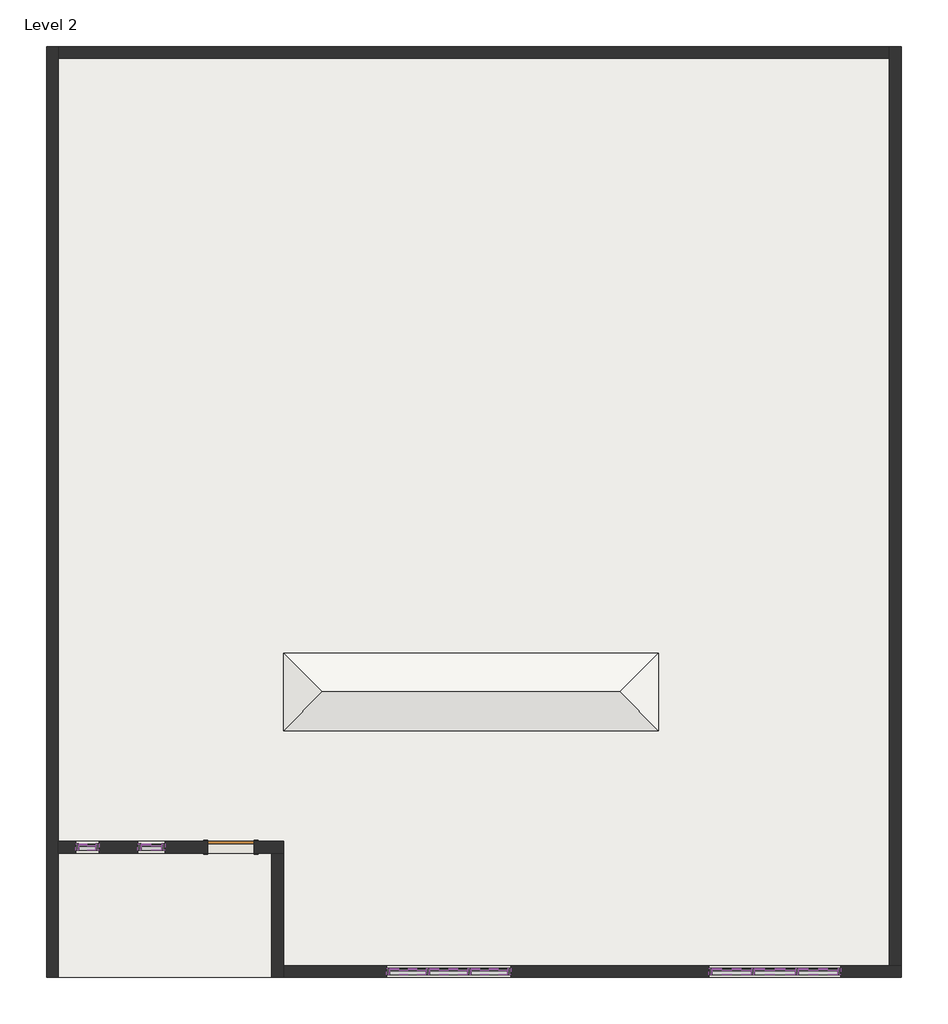
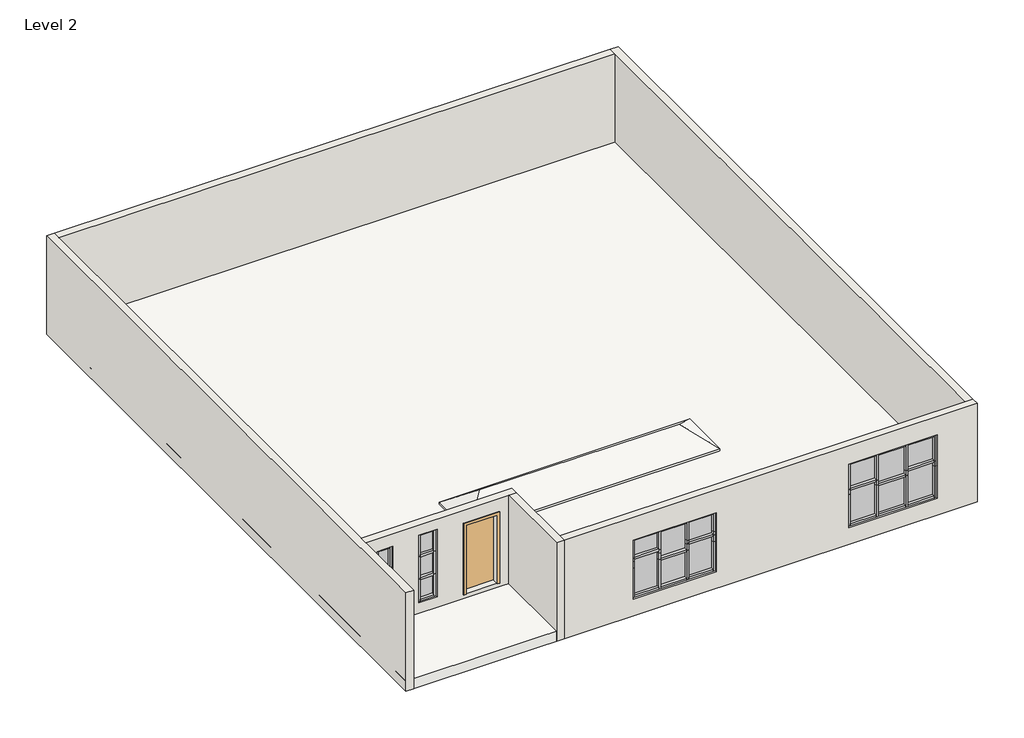
# One storey: 66 members, 18 plates, 6 walls, 2 roofs, 1 door.
"""IFC4 building model written with IfcOpenShell, lengths in millimetres."""

from ifc_helpers import new_model, si_unit, frame, origin, place, context, project, spatial, polyline, outline, extrude, faceted_brep, transform, mapped, element, save
from components import door_0ca8825f, member_ff9f2d30, member_0c1408be, member_7007ad49, member_abeaf8ac, member_9d02be77, member_798d6cad, member_f6f0dfdd, member_876f8f00, member_418a0375, member_7cfea1b5, member_90c805a2, member_80b47cb0, member_0b6e4484, member_4d11dfbc, member_589dede6, member_5e78fce7, member_cffb459a, member_c9167585, member_da94038d, member_275f0c90, member_171fbd6b, member_46f5bc36, member_7d5d45fc, member_9b02ea12, member_d36207d9, member_cfa99961, member_eb4ec5b9, member_8d384f73, system_panel_glazed_68d54f83, system_panel_glazed_d4755e25, system_panel_glazed_0c192b01, system_panel_glazed_dee09a0e, system_panel_glazed_ce1d5741, system_panel_glazed_66e670ab, system_panel_glazed_3c8ea7cb, system_panel_glazed_e6cace74, system_panel_glazed_91241e07, system_panel_glazed_eced71b2, system_panel_glazed_8f137235, system_panel_glazed_21a2a3f6, system_panel_glazed_4e21c323, system_panel_glazed_5de3b49f

model = new_model("IFC4")

# Units and contexts
model_context = context("Model", 3, world=origin())
ifc_project = project(units=[si_unit("LENGTHUNIT", "METRE", prefix="MILLI")], contexts=[model_context])

# Site, building, storey
site = spatial("IfcSite", under=ifc_project)
building = spatial("IfcBuilding", under=site)
storey = spatial("IfcBuildingStorey", under=building, Name="Level 2", Elevation=3048.0)

# Door
placement = place(None, origin())
door_shape = door_0ca8825f(model_context)
element("IfcDoor", 1, ObjectType="Single-Flush : 36\" x 84\"", at=placement, inside=storey, context=model_context, shape_type="MappedRepresentation", body=[
    mapped(door_shape, transform((608.939189, -10823.7602599, 3479.8), x_axis=(1.0, 0.0, 0.0), y_axis=(0.0, 1.0, 0.0), z_axis=(0.0, 0.0, 1.0))),
])

# Members
member_shape = member_ff9f2d30(model_context)
element("IfcMember", 2, ObjectType="Rectangular Mullion : 2.5\" x 5\" rectangular", at=placement, inside=storey, context=model_context, shape_type="MappedRepresentation", body=[
    mapped(member_shape, transform((-2045.360811, -10823.7602599, 5692.5645868), x_axis=(0.0, 0.0, 1.0), y_axis=(0.0, -1.0, 0.0), z_axis=(1.0, 0.0, 0.0))),
])
element("IfcMember", 3, ObjectType="Rectangular Mullion : 2.5\" x 5\" rectangular", at=placement, inside=storey, context=model_context, shape_type="MappedRepresentation", body=[
    mapped(member_shape, transform((-2375.560811, -10823.7602599, 3695.8118947), x_axis=(0.0, 0.0, -1.0), y_axis=(0.0, -1.0, 0.0), z_axis=(-1.0, 0.0, 0.0))),
])
member_2_shape = member_0c1408be(model_context)
element("IfcMember", 4, ObjectType="Rectangular Mullion : 2.5\" x 5\" rectangular", at=placement, inside=storey, context=model_context, shape_type="MappedRepresentation", body=[
    mapped(member_2_shape, transform((-2045.360811, -10823.7602599, 5026.9803561), x_axis=(0.0, 0.0, 1.0), y_axis=(0.0, -1.0, 0.0), z_axis=(1.0, 0.0, 0.0))),
])
element("IfcMember", 5, ObjectType="Rectangular Mullion : 2.5\" x 5\" rectangular", at=placement, inside=storey, context=model_context, shape_type="MappedRepresentation", body=[
    mapped(member_2_shape, transform((-2045.360811, -10823.7602599, 4361.3961254), x_axis=(0.0, 0.0, 1.0), y_axis=(0.0, -1.0, 0.0), z_axis=(1.0, 0.0, 0.0))),
])
member_3_shape = member_7007ad49(model_context)
element("IfcMember", 6, ObjectType="Rectangular Mullion : 2.5\" x 5\" rectangular", at=placement, inside=storey, context=model_context, shape_type="MappedRepresentation", body=[
    mapped(member_3_shape, transform((4437.989189, -13262.1602599, 5393.2664984), x_axis=(0.0, 0.0, 1.0), y_axis=(0.0, -1.0, 0.0), z_axis=(1.0, 0.0, 0.0))),
])
element("IfcMember", 7, ObjectType="Rectangular Mullion : 2.5\" x 5\" rectangular", at=placement, inside=storey, context=model_context, shape_type="MappedRepresentation", body=[
    mapped(member_3_shape, transform((6031.839189, -13262.1602599, 5393.2664984), x_axis=(0.0, 0.0, 1.0), y_axis=(0.0, -1.0, 0.0), z_axis=(1.0, 0.0, 0.0))),
])
element("IfcMember", 8, ObjectType="Rectangular Mullion : 2.5\" x 5\" rectangular", at=placement, inside=storey, context=model_context, shape_type="MappedRepresentation", body=[
    mapped(member_3_shape, transform((5314.289189, -13262.1602599, 3565.6673843), x_axis=(0.0, 0.0, -1.0), y_axis=(0.0, -1.0, 0.0), z_axis=(-1.0, 0.0, 0.0))),
])
element("IfcMember", 9, ObjectType="Rectangular Mullion : 2.5\" x 5\" rectangular", at=placement, inside=storey, context=model_context, shape_type="MappedRepresentation", body=[
    mapped(member_3_shape, transform((3720.439189, -13262.1602599, 3565.6673843), x_axis=(0.0, 0.0, -1.0), y_axis=(0.0, -1.0, 0.0), z_axis=(-1.0, 0.0, 0.0))),
])
member_4_shape = member_abeaf8ac(model_context)
element("IfcMember", 10, ObjectType="Rectangular Mullion : 2.5\" x 5\" rectangular", at=placement, inside=storey, context=model_context, shape_type="MappedRepresentation", body=[
    mapped(member_4_shape, transform((4437.989189, -13262.1602599, 4784.0667937), x_axis=(0.0, 0.0, 1.0), y_axis=(0.0, -1.0, 0.0), z_axis=(1.0, 0.0, 0.0))),
])
element("IfcMember", 11, ObjectType="Rectangular Mullion : 2.5\" x 5\" rectangular", at=placement, inside=storey, context=model_context, shape_type="MappedRepresentation", body=[
    mapped(member_4_shape, transform((6031.839189, -13262.1602599, 4682.5335096), x_axis=(0.0, 0.0, 1.0), y_axis=(0.0, -1.0, 0.0), z_axis=(1.0, 0.0, 0.0))),
])
member_5_shape = member_9d02be77(model_context)
element("IfcMember", 12, ObjectType="Rectangular Mullion : 2.5\" x 5\" rectangular", at=placement, inside=storey, context=model_context, shape_type="MappedRepresentation", body=[
    mapped(member_5_shape, transform((5250.789189, -13262.1602599, 5393.2664984), x_axis=(0.0, 0.0, 1.0), y_axis=(0.0, -1.0, 0.0), z_axis=(1.0, 0.0, 0.0))),
])
element("IfcMember", 13, ObjectType="Rectangular Mullion : 2.5\" x 5\" rectangular", at=placement, inside=storey, context=model_context, shape_type="MappedRepresentation", body=[
    mapped(member_5_shape, transform((4501.489189, -13262.1602599, 3565.6673843), x_axis=(0.0, 0.0, -1.0), y_axis=(0.0, -1.0, 0.0), z_axis=(-1.0, 0.0, 0.0))),
])
member_6_shape = member_798d6cad(model_context)
element("IfcMember", 14, ObjectType="Rectangular Mullion : 2.5\" x 5\" rectangular", at=placement, inside=storey, context=model_context, shape_type="MappedRepresentation", body=[
    mapped(member_6_shape, transform((5250.789189, -13262.1602599, 4479.4669413), x_axis=(0.0, 0.0, 1.0), y_axis=(0.0, -1.0, 0.0), z_axis=(1.0, 0.0, 0.0))),
])
member_7_shape = member_f6f0dfdd(model_context)
element("IfcMember", 15, ObjectType="Rectangular Mullion : 2.5\" x 5\" rectangular", at=placement, inside=storey, context=model_context, shape_type="MappedRepresentation", body=[
    mapped(member_7_shape, transform((10845.139189, -13262.1602599, 4552.2497508), x_axis=(1.0, 0.0, 0.0), y_axis=(0.0, -1.0, 0.0), z_axis=(0.0, 0.0, -1.0))),
])
element("IfcMember", 16, ObjectType="Rectangular Mullion : 2.5\" x 5\" rectangular", at=placement, inside=storey, context=model_context, shape_type="MappedRepresentation", body=[
    mapped(member_7_shape, transform((11708.739189, -13262.1602599, 4552.2497508), x_axis=(1.0, 0.0, 0.0), y_axis=(0.0, -1.0, 0.0), z_axis=(0.0, 0.0, -1.0))),
])
member_8_shape = member_876f8f00(model_context)
element("IfcMember", 17, ObjectType="Rectangular Mullion : 2.5\" x 5\" rectangular", at=placement, inside=storey, context=model_context, shape_type="MappedRepresentation", body=[
    mapped(member_8_shape, transform((12572.339189, -13262.1602599, 4552.2497508), x_axis=(1.0, 0.0, 0.0), y_axis=(0.0, -1.0, 0.0), z_axis=(0.0, 0.0, -1.0))),
])
member_9_shape = member_418a0375(model_context)
element("IfcMember", 18, ObjectType="Rectangular Mullion : 2.5\" x 5\" rectangular", at=placement, inside=storey, context=model_context, shape_type="MappedRepresentation", body=[
    mapped(member_9_shape, transform((-2439.060811, -10823.7602599, 5692.5645868), x_axis=(-1.0, 0.0, 0.0), y_axis=(0.0, -1.0, 0.0), z_axis=(0.0, 0.0, 1.0))),
])
element("IfcMember", 19, ObjectType="Rectangular Mullion : 2.5\" x 5\" rectangular", at=placement, inside=storey, context=model_context, shape_type="MappedRepresentation", body=[
    mapped(member_9_shape, transform((-1981.860811, -10823.7602599, 5026.9803561), x_axis=(1.0, 0.0, 0.0), y_axis=(0.0, -1.0, 0.0), z_axis=(0.0, 0.0, -1.0))),
])
element("IfcMember", 20, ObjectType="Rectangular Mullion : 2.5\" x 5\" rectangular", at=placement, inside=storey, context=model_context, shape_type="MappedRepresentation", body=[
    mapped(member_9_shape, transform((-2439.060811, -10823.7602599, 5026.9803561), x_axis=(-1.0, 0.0, 0.0), y_axis=(0.0, -1.0, 0.0), z_axis=(0.0, 0.0, 1.0))),
])
element("IfcMember", 21, ObjectType="Rectangular Mullion : 2.5\" x 5\" rectangular", at=placement, inside=storey, context=model_context, shape_type="MappedRepresentation", body=[
    mapped(member_9_shape, transform((-1981.860811, -10823.7602599, 4361.3961254), x_axis=(1.0, 0.0, 0.0), y_axis=(0.0, -1.0, 0.0), z_axis=(0.0, 0.0, -1.0))),
])
element("IfcMember", 22, ObjectType="Rectangular Mullion : 2.5\" x 5\" rectangular", at=placement, inside=storey, context=model_context, shape_type="MappedRepresentation", body=[
    mapped(member_9_shape, transform((-2439.060811, -10823.7602599, 4361.3961254), x_axis=(-1.0, 0.0, 0.0), y_axis=(0.0, -1.0, 0.0), z_axis=(0.0, 0.0, 1.0))),
])
element("IfcMember", 23, ObjectType="Rectangular Mullion : 2.5\" x 5\" rectangular", at=placement, inside=storey, context=model_context, shape_type="MappedRepresentation", body=[
    mapped(member_9_shape, transform((-1981.860811, -10823.7602599, 3695.8118947), x_axis=(1.0, 0.0, 0.0), y_axis=(0.0, -1.0, 0.0), z_axis=(0.0, 0.0, -1.0))),
])
member_10_shape = member_7cfea1b5(model_context)
element("IfcMember", 24, ObjectType="Rectangular Mullion : 2.5\" x 5\" rectangular", at=placement, inside=storey, context=model_context, shape_type="MappedRepresentation", body=[
    mapped(member_10_shape, transform((-749.960811, -10823.7602599, 5778.2338442), x_axis=(0.0, 0.0, 1.0), y_axis=(0.0, -1.0, 0.0), z_axis=(1.0, 0.0, 0.0))),
])
element("IfcMember", 25, ObjectType="Rectangular Mullion : 2.5\" x 5\" rectangular", at=placement, inside=storey, context=model_context, shape_type="MappedRepresentation", body=[
    mapped(member_10_shape, transform((-1156.360811, -10823.7602599, 3676.0420661), x_axis=(0.0, 0.0, -1.0), y_axis=(0.0, -1.0, 0.0), z_axis=(-1.0, 0.0, 0.0))),
])
member_11_shape = member_90c805a2(model_context)
element("IfcMember", 26, ObjectType="Rectangular Mullion : 2.5\" x 5\" rectangular", at=placement, inside=storey, context=model_context, shape_type="MappedRepresentation", body=[
    mapped(member_11_shape, transform((-749.960811, -10823.7602599, 4376.7726588), x_axis=(0.0, 0.0, 1.0), y_axis=(0.0, -1.0, 0.0), z_axis=(1.0, 0.0, 0.0))),
])
element("IfcMember", 27, ObjectType="Rectangular Mullion : 2.5\" x 5\" rectangular", at=placement, inside=storey, context=model_context, shape_type="MappedRepresentation", body=[
    mapped(member_11_shape, transform((-749.960811, -10823.7602599, 5077.5032515), x_axis=(0.0, 0.0, 1.0), y_axis=(0.0, -1.0, 0.0), z_axis=(1.0, 0.0, 0.0))),
])
member_12_shape = member_80b47cb0(model_context)
element("IfcMember", 28, ObjectType="Rectangular Mullion : 2.5\" x 5\" rectangular", at=placement, inside=storey, context=model_context, shape_type="MappedRepresentation", body=[
    mapped(member_12_shape, transform((-1219.860811, -10823.7602599, 4376.7726588), x_axis=(-1.0, 0.0, 0.0), y_axis=(0.0, -1.0, 0.0), z_axis=(0.0, 0.0, 1.0))),
])
element("IfcMember", 29, ObjectType="Rectangular Mullion : 2.5\" x 5\" rectangular", at=placement, inside=storey, context=model_context, shape_type="MappedRepresentation", body=[
    mapped(member_12_shape, transform((-686.460811, -10823.7602599, 3676.0420661), x_axis=(1.0, 0.0, 0.0), y_axis=(0.0, -1.0, 0.0), z_axis=(0.0, 0.0, -1.0))),
])
element("IfcMember", 30, ObjectType="Rectangular Mullion : 2.5\" x 5\" rectangular", at=placement, inside=storey, context=model_context, shape_type="MappedRepresentation", body=[
    mapped(member_12_shape, transform((-1219.860811, -10823.7602599, 5077.5032515), x_axis=(-1.0, 0.0, 0.0), y_axis=(0.0, -1.0, 0.0), z_axis=(0.0, 0.0, 1.0))),
])
element("IfcMember", 31, ObjectType="Rectangular Mullion : 2.5\" x 5\" rectangular", at=placement, inside=storey, context=model_context, shape_type="MappedRepresentation", body=[
    mapped(member_12_shape, transform((-1219.860811, -10823.7602599, 5778.2338442), x_axis=(-1.0, 0.0, 0.0), y_axis=(0.0, -1.0, 0.0), z_axis=(0.0, 0.0, 1.0))),
])
element("IfcMember", 32, ObjectType="Rectangular Mullion : 2.5\" x 5\" rectangular", at=placement, inside=storey, context=model_context, shape_type="MappedRepresentation", body=[
    mapped(member_12_shape, transform((-686.460811, -10823.7602599, 4376.7726588), x_axis=(1.0, 0.0, 0.0), y_axis=(0.0, -1.0, 0.0), z_axis=(0.0, 0.0, -1.0))),
])
element("IfcMember", 33, ObjectType="Rectangular Mullion : 2.5\" x 5\" rectangular", at=placement, inside=storey, context=model_context, shape_type="MappedRepresentation", body=[
    mapped(member_12_shape, transform((-686.460811, -10823.7602599, 5077.5032515), x_axis=(1.0, 0.0, 0.0), y_axis=(0.0, -1.0, 0.0), z_axis=(0.0, 0.0, -1.0))),
])
member_13_shape = member_0b6e4484(model_context)
element("IfcMember", 34, ObjectType="Rectangular Mullion : 2.5\" x 5\" rectangular", at=placement, inside=storey, context=model_context, shape_type="MappedRepresentation", body=[
    mapped(member_13_shape, transform((3656.939189, -13262.1602599, 4682.5335096), x_axis=(-1.0, 0.0, 0.0), y_axis=(0.0, -1.0, 0.0), z_axis=(0.0, 0.0, 1.0))),
])
member_14_shape = member_4d11dfbc(model_context)
element("IfcMember", 35, ObjectType="Rectangular Mullion : 2.5\" x 5\" rectangular", at=placement, inside=storey, context=model_context, shape_type="MappedRepresentation", body=[
    mapped(member_14_shape, transform((3656.939189, -13262.1602599, 4784.0667937), x_axis=(-1.0, 0.0, 0.0), y_axis=(0.0, -1.0, 0.0), z_axis=(0.0, 0.0, 1.0))),
])
member_15_shape = member_589dede6(model_context)
element("IfcMember", 36, ObjectType="Rectangular Mullion : 2.5\" x 5\" rectangular", at=placement, inside=storey, context=model_context, shape_type="MappedRepresentation", body=[
    mapped(member_15_shape, transform((3656.939189, -13262.1602599, 5393.2664984), x_axis=(-1.0, 0.0, 0.0), y_axis=(0.0, -1.0, 0.0), z_axis=(0.0, 0.0, 1.0))),
])
member_16_shape = member_5e78fce7(model_context)
element("IfcMember", 37, ObjectType="Rectangular Mullion : 2.5\" x 5\" rectangular", at=placement, inside=storey, context=model_context, shape_type="MappedRepresentation", body=[
    mapped(member_16_shape, transform((4469.739189, -13262.1602599, 4682.5335096), x_axis=(1.0, 0.0, 0.0), y_axis=(0.0, -1.0, 0.0), z_axis=(0.0, 0.0, -1.0))),
])
member_17_shape = member_cffb459a(model_context)
element("IfcMember", 38, ObjectType="Rectangular Mullion : 2.5\" x 5\" rectangular", at=placement, inside=storey, context=model_context, shape_type="MappedRepresentation", body=[
    mapped(member_17_shape, transform((4469.739189, -13262.1602599, 4784.0667937), x_axis=(1.0, 0.0, 0.0), y_axis=(0.0, -1.0, 0.0), z_axis=(0.0, 0.0, -1.0))),
])
member_18_shape = member_c9167585(model_context)
element("IfcMember", 39, ObjectType="Rectangular Mullion : 2.5\" x 5\" rectangular", at=placement, inside=storey, context=model_context, shape_type="MappedRepresentation", body=[
    mapped(member_18_shape, transform((3656.939189, -13262.1602599, 4479.4669413), x_axis=(-1.0, 0.0, 0.0), y_axis=(0.0, -1.0, 0.0), z_axis=(0.0, 0.0, 1.0))),
])
member_19_shape = member_da94038d(model_context)
element("IfcMember", 40, ObjectType="Rectangular Mullion : 2.5\" x 5\" rectangular", at=placement, inside=storey, context=model_context, shape_type="MappedRepresentation", body=[
    mapped(member_19_shape, transform((4469.739189, -13262.1602599, 4479.4669413), x_axis=(1.0, 0.0, 0.0), y_axis=(0.0, -1.0, 0.0), z_axis=(0.0, 0.0, -1.0))),
])
member_20_shape = member_275f0c90(model_context)
element("IfcMember", 41, ObjectType="Rectangular Mullion : 2.5\" x 5\" rectangular", at=placement, inside=storey, context=model_context, shape_type="MappedRepresentation", body=[
    mapped(member_20_shape, transform((4469.739189, -13262.1602599, 3565.6673843), x_axis=(1.0, 0.0, 0.0), y_axis=(0.0, -1.0, 0.0), z_axis=(0.0, 0.0, -1.0))),
])
element("IfcMember", 42, ObjectType="Rectangular Mullion : 2.5\" x 5\" rectangular", at=placement, inside=storey, context=model_context, shape_type="MappedRepresentation", body=[
    mapped(member_20_shape, transform((5282.539189, -13262.1602599, 3565.6673843), x_axis=(1.0, 0.0, 0.0), y_axis=(0.0, -1.0, 0.0), z_axis=(0.0, 0.0, -1.0))),
])
element("IfcMember", 43, ObjectType="Rectangular Mullion : 2.5\" x 5\" rectangular", at=placement, inside=storey, context=model_context, shape_type="MappedRepresentation", body=[
    mapped(member_17_shape, transform((5282.539189, -13262.1602599, 4784.0667937), x_axis=(1.0, 0.0, 0.0), y_axis=(0.0, -1.0, 0.0), z_axis=(0.0, 0.0, -1.0))),
])
element("IfcMember", 44, ObjectType="Rectangular Mullion : 2.5\" x 5\" rectangular", at=placement, inside=storey, context=model_context, shape_type="MappedRepresentation", body=[
    mapped(member_16_shape, transform((5282.539189, -13262.1602599, 4682.5335096), x_axis=(1.0, 0.0, 0.0), y_axis=(0.0, -1.0, 0.0), z_axis=(0.0, 0.0, -1.0))),
])
element("IfcMember", 45, ObjectType="Rectangular Mullion : 2.5\" x 5\" rectangular", at=placement, inside=storey, context=model_context, shape_type="MappedRepresentation", body=[
    mapped(member_19_shape, transform((5282.539189, -13262.1602599, 4479.4669413), x_axis=(1.0, 0.0, 0.0), y_axis=(0.0, -1.0, 0.0), z_axis=(0.0, 0.0, -1.0))),
])
element("IfcMember", 46, ObjectType="Rectangular Mullion : 2.5\" x 5\" rectangular", at=placement, inside=storey, context=model_context, shape_type="MappedRepresentation", body=[
    mapped(member_14_shape, transform((6095.339189, -13262.1602599, 4682.5335096), x_axis=(1.0, 0.0, 0.0), y_axis=(0.0, -1.0, 0.0), z_axis=(0.0, 0.0, -1.0))),
])
element("IfcMember", 47, ObjectType="Rectangular Mullion : 2.5\" x 5\" rectangular", at=placement, inside=storey, context=model_context, shape_type="MappedRepresentation", body=[
    mapped(member_15_shape, transform((6095.339189, -13262.1602599, 4784.0667937), x_axis=(1.0, 0.0, 0.0), y_axis=(0.0, -1.0, 0.0), z_axis=(0.0, 0.0, -1.0))),
])
element("IfcMember", 48, ObjectType="Rectangular Mullion : 2.5\" x 5\" rectangular", at=placement, inside=storey, context=model_context, shape_type="MappedRepresentation", body=[
    mapped(member_13_shape, transform((6095.339189, -13262.1602599, 4479.4669413), x_axis=(1.0, 0.0, 0.0), y_axis=(0.0, -1.0, 0.0), z_axis=(0.0, 0.0, -1.0))),
])
element("IfcMember", 49, ObjectType="Rectangular Mullion : 2.5\" x 5\" rectangular", at=placement, inside=storey, context=model_context, shape_type="MappedRepresentation", body=[
    mapped(member_18_shape, transform((6095.339189, -13262.1602599, 3565.6673843), x_axis=(1.0, 0.0, 0.0), y_axis=(0.0, -1.0, 0.0), z_axis=(0.0, 0.0, -1.0))),
])
element("IfcMember", 50, ObjectType="Rectangular Mullion : 2.5\" x 5\" rectangular", at=placement, inside=storey, context=model_context, shape_type="MappedRepresentation", body=[
    mapped(member_8_shape, transform((9981.539189, -13262.1602599, 4704.6497508), x_axis=(-1.0, 0.0, 0.0), y_axis=(0.0, -1.0, 0.0), z_axis=(0.0, 0.0, 1.0))),
])
member_21_shape = member_171fbd6b(model_context)
element("IfcMember", 51, ObjectType="Rectangular Mullion : 2.5\" x 5\" rectangular", at=placement, inside=storey, context=model_context, shape_type="MappedRepresentation", body=[
    mapped(member_21_shape, transform((9981.539189, -13262.1602599, 5535.3242495), x_axis=(-1.0, 0.0, 0.0), y_axis=(0.0, -1.0, 0.0), z_axis=(0.0, 0.0, 1.0))),
])
member_22_shape = member_46f5bc36(model_context)
element("IfcMember", 52, ObjectType="Rectangular Mullion : 2.5\" x 5\" rectangular", at=placement, inside=storey, context=model_context, shape_type="MappedRepresentation", body=[
    mapped(member_22_shape, transform((10813.389189, -13262.1602599, 5535.3242495), x_axis=(0.0, 0.0, 1.0), y_axis=(0.0, -1.0, 0.0), z_axis=(1.0, 0.0, 0.0))),
])
element("IfcMember", 53, ObjectType="Rectangular Mullion : 2.5\" x 5\" rectangular", at=placement, inside=storey, context=model_context, shape_type="MappedRepresentation", body=[
    mapped(member_22_shape, transform((12508.839189, -13262.1602599, 5535.3242495), x_axis=(0.0, 0.0, 1.0), y_axis=(0.0, -1.0, 0.0), z_axis=(1.0, 0.0, 0.0))),
])
member_23_shape = member_7d5d45fc(model_context)
element("IfcMember", 54, ObjectType="Rectangular Mullion : 2.5\" x 5\" rectangular", at=placement, inside=storey, context=model_context, shape_type="MappedRepresentation", body=[
    mapped(member_23_shape, transform((12508.839189, -13262.1602599, 4704.6497508), x_axis=(0.0, 0.0, 1.0), y_axis=(0.0, -1.0, 0.0), z_axis=(1.0, 0.0, 0.0))),
])
element("IfcMember", 55, ObjectType="Rectangular Mullion : 2.5\" x 5\" rectangular", at=placement, inside=storey, context=model_context, shape_type="MappedRepresentation", body=[
    mapped(member_23_shape, transform((10813.389189, -13262.1602599, 4704.6497508), x_axis=(0.0, 0.0, 1.0), y_axis=(0.0, -1.0, 0.0), z_axis=(1.0, 0.0, 0.0))),
])
member_24_shape = member_9b02ea12(model_context)
element("IfcMember", 56, ObjectType="Rectangular Mullion : 2.5\" x 5\" rectangular", at=placement, inside=storey, context=model_context, shape_type="MappedRepresentation", body=[
    mapped(member_24_shape, transform((10845.139189, -13262.1602599, 4704.6497508), x_axis=(1.0, 0.0, 0.0), y_axis=(0.0, -1.0, 0.0), z_axis=(0.0, 0.0, -1.0))),
])
element("IfcMember", 57, ObjectType="Rectangular Mullion : 2.5\" x 5\" rectangular", at=placement, inside=storey, context=model_context, shape_type="MappedRepresentation", body=[
    mapped(member_24_shape, transform((11708.739189, -13262.1602599, 4704.6497508), x_axis=(1.0, 0.0, 0.0), y_axis=(0.0, -1.0, 0.0), z_axis=(0.0, 0.0, -1.0))),
])
member_25_shape = member_d36207d9(model_context)
element("IfcMember", 58, ObjectType="Rectangular Mullion : 2.5\" x 5\" rectangular", at=placement, inside=storey, context=model_context, shape_type="MappedRepresentation", body=[
    mapped(member_25_shape, transform((11676.989189, -13262.1602599, 5535.3242495), x_axis=(0.0, 0.0, 1.0), y_axis=(0.0, -1.0, 0.0), z_axis=(1.0, 0.0, 0.0))),
])
member_26_shape = member_cfa99961(model_context)
element("IfcMember", 59, ObjectType="Rectangular Mullion : 2.5\" x 5\" rectangular", at=placement, inside=storey, context=model_context, shape_type="MappedRepresentation", body=[
    mapped(member_26_shape, transform((11676.989189, -13262.1602599, 4552.2497508), x_axis=(0.0, 0.0, 1.0), y_axis=(0.0, -1.0, 0.0), z_axis=(1.0, 0.0, 0.0))),
])
element("IfcMember", 60, ObjectType="Rectangular Mullion : 2.5\" x 5\" rectangular", at=placement, inside=storey, context=model_context, shape_type="MappedRepresentation", body=[
    mapped(member_21_shape, transform((12572.339189, -13262.1602599, 4704.6497508), x_axis=(1.0, 0.0, 0.0), y_axis=(0.0, -1.0, 0.0), z_axis=(0.0, 0.0, -1.0))),
])
member_27_shape = member_eb4ec5b9(model_context)
element("IfcMember", 61, ObjectType="Rectangular Mullion : 2.5\" x 5\" rectangular", at=placement, inside=storey, context=model_context, shape_type="MappedRepresentation", body=[
    mapped(member_27_shape, transform((10845.139189, -13262.1602599, 3569.1752521), x_axis=(1.0, 0.0, 0.0), y_axis=(0.0, -1.0, 0.0), z_axis=(0.0, 0.0, -1.0))),
])
element("IfcMember", 62, ObjectType="Rectangular Mullion : 2.5\" x 5\" rectangular", at=placement, inside=storey, context=model_context, shape_type="MappedRepresentation", body=[
    mapped(member_27_shape, transform((11708.739189, -13262.1602599, 3569.1752521), x_axis=(1.0, 0.0, 0.0), y_axis=(0.0, -1.0, 0.0), z_axis=(0.0, 0.0, -1.0))),
])
element("IfcMember", 63, ObjectType="Rectangular Mullion : 2.5\" x 5\" rectangular", at=placement, inside=storey, context=model_context, shape_type="MappedRepresentation", body=[
    mapped(member_22_shape, transform((11740.489189, -13262.1602599, 3569.1752521), x_axis=(0.0, 0.0, -1.0), y_axis=(0.0, -1.0, 0.0), z_axis=(-1.0, 0.0, 0.0))),
])
element("IfcMember", 64, ObjectType="Rectangular Mullion : 2.5\" x 5\" rectangular", at=placement, inside=storey, context=model_context, shape_type="MappedRepresentation", body=[
    mapped(member_22_shape, transform((10045.039189, -13262.1602599, 3569.1752521), x_axis=(0.0, 0.0, -1.0), y_axis=(0.0, -1.0, 0.0), z_axis=(-1.0, 0.0, 0.0))),
])
element("IfcMember", 65, ObjectType="Rectangular Mullion : 2.5\" x 5\" rectangular", at=placement, inside=storey, context=model_context, shape_type="MappedRepresentation", body=[
    mapped(member_25_shape, transform((10876.889189, -13262.1602599, 3569.1752521), x_axis=(0.0, 0.0, -1.0), y_axis=(0.0, -1.0, 0.0), z_axis=(-1.0, 0.0, 0.0))),
])
member_28_shape = member_8d384f73(model_context)
element("IfcMember", 66, ObjectType="Rectangular Mullion : 2.5\" x 5\" rectangular", at=placement, inside=storey, context=model_context, shape_type="MappedRepresentation", body=[
    mapped(member_28_shape, transform((9981.539189, -13262.1602599, 4552.2497508), x_axis=(-1.0, 0.0, 0.0), y_axis=(0.0, -1.0, 0.0), z_axis=(0.0, 0.0, 1.0))),
])
element("IfcMember", 67, ObjectType="Rectangular Mullion : 2.5\" x 5\" rectangular", at=placement, inside=storey, context=model_context, shape_type="MappedRepresentation", body=[
    mapped(member_28_shape, transform((12572.339189, -13262.1602599, 3569.1752521), x_axis=(1.0, 0.0, 0.0), y_axis=(0.0, -1.0, 0.0), z_axis=(0.0, 0.0, -1.0))),
])

# Plates
system_panel_glazed_shape = system_panel_glazed_68d54f83(model_context)
element("IfcPlate", 68, ObjectType="System Panel : Glazed", at=placement, inside=storey, context=model_context, shape_type="MappedRepresentation", body=[
    mapped(system_panel_glazed_shape, transform((-2210.460811, -10823.7602599, 3759.3118947), x_axis=(1.0, 0.0, 0.0), y_axis=(0.0, 1.0, 0.0), z_axis=(0.0, 0.0, 1.0))),
])
element("IfcPlate", 69, ObjectType="System Panel : Glazed", at=placement, inside=storey, context=model_context, shape_type="MappedRepresentation", body=[
    mapped(system_panel_glazed_shape, transform((-2210.460811, -10823.7602599, 5058.7303561), x_axis=(1.0, 0.0, 0.0), y_axis=(0.0, 1.0, 0.0), z_axis=(0.0, 0.0, 1.0))),
])
system_panel_glazed_2_shape = system_panel_glazed_d4755e25(model_context)
element("IfcPlate", 70, ObjectType="System Panel : Glazed", at=placement, inside=storey, context=model_context, shape_type="MappedRepresentation", body=[
    mapped(system_panel_glazed_2_shape, transform((-2210.460811, -10823.7602599, 4393.1461254), x_axis=(1.0, 0.0, 0.0), y_axis=(0.0, 1.0, 0.0), z_axis=(0.0, 0.0, 1.0))),
])
system_panel_glazed_3_shape = system_panel_glazed_0c192b01(model_context)
element("IfcPlate", 71, ObjectType="System Panel : Glazed", at=placement, inside=storey, context=model_context, shape_type="MappedRepresentation", body=[
    mapped(system_panel_glazed_3_shape, transform((-953.160811, -10823.7602599, 4408.5226588), x_axis=(1.0, 0.0, 0.0), y_axis=(0.0, 1.0, 0.0), z_axis=(0.0, 0.0, 1.0))),
])
system_panel_glazed_4_shape = system_panel_glazed_dee09a0e(model_context)
element("IfcPlate", 72, ObjectType="System Panel : Glazed", at=placement, inside=storey, context=model_context, shape_type="MappedRepresentation", body=[
    mapped(system_panel_glazed_4_shape, transform((-953.160811, -10823.7602599, 3739.5420661), x_axis=(1.0, 0.0, 0.0), y_axis=(0.0, 1.0, 0.0), z_axis=(0.0, 0.0, 1.0))),
])
element("IfcPlate", 73, ObjectType="System Panel : Glazed", at=placement, inside=storey, context=model_context, shape_type="MappedRepresentation", body=[
    mapped(system_panel_glazed_4_shape, transform((-953.160811, -10823.7602599, 5109.2532515), x_axis=(1.0, 0.0, 0.0), y_axis=(0.0, 1.0, 0.0), z_axis=(0.0, 0.0, 1.0))),
])
system_panel_glazed_5_shape = system_panel_glazed_ce1d5741(model_context)
element("IfcPlate", 74, ObjectType="System Panel : Glazed", at=placement, inside=storey, context=model_context, shape_type="MappedRepresentation", body=[
    mapped(system_panel_glazed_5_shape, transform((4079.214189, -13262.1602599, 4815.8167937), x_axis=(1.0, 0.0, 0.0), y_axis=(0.0, 1.0, 0.0), z_axis=(0.0, 0.0, 1.0))),
])
system_panel_glazed_6_shape = system_panel_glazed_66e670ab(model_context)
element("IfcPlate", 75, ObjectType="System Panel : Glazed", at=placement, inside=storey, context=model_context, shape_type="MappedRepresentation", body=[
    mapped(system_panel_glazed_6_shape, transform((4079.214189, -13262.1602599, 3629.1673843), x_axis=(1.0, 0.0, 0.0), y_axis=(0.0, 1.0, 0.0), z_axis=(0.0, 0.0, 1.0))),
])
system_panel_glazed_7_shape = system_panel_glazed_3c8ea7cb(model_context)
element("IfcPlate", 76, ObjectType="System Panel : Glazed", at=placement, inside=storey, context=model_context, shape_type="MappedRepresentation", body=[
    mapped(system_panel_glazed_7_shape, transform((4876.139189, -13262.1602599, 3629.1673843), x_axis=(1.0, 0.0, 0.0), y_axis=(0.0, 1.0, 0.0), z_axis=(0.0, 0.0, 1.0))),
])
system_panel_glazed_8_shape = system_panel_glazed_e6cace74(model_context)
element("IfcPlate", 77, ObjectType="System Panel : Glazed", at=placement, inside=storey, context=model_context, shape_type="MappedRepresentation", body=[
    mapped(system_panel_glazed_8_shape, transform((4876.139189, -13262.1602599, 4511.2169413), x_axis=(1.0, 0.0, 0.0), y_axis=(0.0, 1.0, 0.0), z_axis=(0.0, 0.0, 1.0))),
])
system_panel_glazed_9_shape = system_panel_glazed_91241e07(model_context)
element("IfcPlate", 78, ObjectType="System Panel : Glazed", at=placement, inside=storey, context=model_context, shape_type="MappedRepresentation", body=[
    mapped(system_panel_glazed_9_shape, transform((5673.064189, -13262.1602599, 3629.1673843), x_axis=(1.0, 0.0, 0.0), y_axis=(0.0, 1.0, 0.0), z_axis=(0.0, 0.0, 1.0))),
])
system_panel_glazed_10_shape = system_panel_glazed_eced71b2(model_context)
element("IfcPlate", 79, ObjectType="System Panel : Glazed", at=placement, inside=storey, context=model_context, shape_type="MappedRepresentation", body=[
    mapped(system_panel_glazed_10_shape, transform((5673.064189, -13262.1602599, 4714.2835096), x_axis=(1.0, 0.0, 0.0), y_axis=(0.0, 1.0, 0.0), z_axis=(0.0, 0.0, 1.0))),
])
system_panel_glazed_11_shape = system_panel_glazed_8f137235(model_context)
element("IfcPlate", 80, ObjectType="System Panel : Glazed", at=placement, inside=storey, context=model_context, shape_type="MappedRepresentation", body=[
    mapped(system_panel_glazed_11_shape, transform((10429.214189, -13262.1602599, 4736.3997508), x_axis=(1.0, 0.0, 0.0), y_axis=(0.0, 1.0, 0.0), z_axis=(0.0, 0.0, 1.0))),
])
element("IfcPlate", 81, ObjectType="System Panel : Glazed", at=placement, inside=storey, context=model_context, shape_type="MappedRepresentation", body=[
    mapped(system_panel_glazed_11_shape, transform((12124.664189, -13262.1602599, 4736.3997508), x_axis=(1.0, 0.0, 0.0), y_axis=(0.0, 1.0, 0.0), z_axis=(0.0, 0.0, 1.0))),
])
system_panel_glazed_12_shape = system_panel_glazed_21a2a3f6(model_context)
element("IfcPlate", 82, ObjectType="System Panel : Glazed", at=placement, inside=storey, context=model_context, shape_type="MappedRepresentation", body=[
    mapped(system_panel_glazed_12_shape, transform((11276.939189, -13262.1602599, 4583.9997508), x_axis=(1.0, 0.0, 0.0), y_axis=(0.0, 1.0, 0.0), z_axis=(0.0, 0.0, 1.0))),
])
system_panel_glazed_13_shape = system_panel_glazed_4e21c323(model_context)
element("IfcPlate", 83, ObjectType="System Panel : Glazed", at=placement, inside=storey, context=model_context, shape_type="MappedRepresentation", body=[
    mapped(system_panel_glazed_13_shape, transform((10429.214189, -13262.1602599, 3632.6752521), x_axis=(1.0, 0.0, 0.0), y_axis=(0.0, 1.0, 0.0), z_axis=(0.0, 0.0, 1.0))),
])
element("IfcPlate", 84, ObjectType="System Panel : Glazed", at=placement, inside=storey, context=model_context, shape_type="MappedRepresentation", body=[
    mapped(system_panel_glazed_13_shape, transform((12124.664189, -13262.1602599, 3632.6752521), x_axis=(1.0, 0.0, 0.0), y_axis=(0.0, 1.0, 0.0), z_axis=(0.0, 0.0, 1.0))),
])
system_panel_glazed_14_shape = system_panel_glazed_5de3b49f(model_context)
element("IfcPlate", 85, ObjectType="System Panel : Glazed", at=placement, inside=storey, context=model_context, shape_type="MappedRepresentation", body=[
    mapped(system_panel_glazed_14_shape, transform((11276.939189, -13262.1602599, 3632.6752521), x_axis=(1.0, 0.0, 0.0), y_axis=(0.0, 1.0, 0.0), z_axis=(0.0, 0.0, 1.0))),
])

# Roofs
element("IfcRoof", 86, ObjectType="Generic - 12\"", at=placement, inside=storey, context=model_context, shape_type="SweptSolid", body=[
    extrude(outline(polyline([(-3010.560811, 4873.4397401), (13753.439189, 4873.4397401), (13753.439189, -13376.4602599), (-3010.560811, -13376.4602599), (-3010.560811, 4873.4397401)])), frame((0.0, 0.0, 3048.0), z_axis=(0.0, 0.0, 1.0), x_axis=(1.0, 0.0, 0.0)), (0.0, 0.0, 1.0), 304.8),
])
element("IfcRoof", 87, ObjectType="Generic - 12\"", at=placement, inside=storey, context=model_context, shape_type="Brep", body=[
    faceted_brep([(8234.4532496, -7778.6123124, 3615.3644546), (8990.939189, -8535.0982518, 3048.0), (1637.639189, -8535.0982518, 3048.0), (2394.1251284, -7778.6123124, 3615.3644546), (1637.639189, -7022.1263729, 3048.0), (8990.939189, -7022.1263729, 3048.0), (8990.939189, -8535.0982518, 3429.0), (8234.4532496, -7778.6123124, 3996.3644546), (2394.1251284, -7778.6123124, 3996.3644546), (1637.639189, -8535.0982518, 3429.0), (1637.639189, -7022.1263729, 3429.0), (8990.939189, -7022.1263729, 3429.0)], [[[0, 1, 2, 3]], [[4, 3, 2]], [[5, 0, 3, 4]], [[1, 0, 5]], [[6, 7, 8, 9]], [[10, 9, 8]], [[11, 10, 8, 7]], [[6, 11, 7]], [[5, 11, 6, 1]], [[4, 10, 11, 5]], [[2, 9, 10, 4]], [[1, 6, 9, 2]]]),
])

# Walls
element("IfcWall", 88, ObjectType="9\"", at=placement, inside=storey, context=model_context, shape_type="Brep", body=[
    faceted_brep([(-3010.560811, 4873.4397401, 3048.0), (-3010.560811, -13376.4602599, 3048.0), (-3010.560811, -13376.4602599, 6096.0), (-3010.560811, 4873.4397401, 6096.0), (-2781.960811, 4873.4397401, 3048.0), (-2781.960811, 4873.4397401, 6096.0), (-2781.960811, 4644.8397401, 6096.0), (-2781.960811, -10709.4602599, 6096.0), (-2781.960811, -10938.0602599, 6096.0), (-2781.960811, -13376.4602599, 6096.0), (-2781.960811, -13376.4602599, 3048.0), (-2781.960811, -10938.0602599, 3048.0), (-2781.960811, -10709.4602599, 3048.0), (-2781.960811, 4644.8397401, 3048.0)], [[[0, 1, 2, 3]], [[4, 5, 6, 7, 8, 9, 10, 11, 12, 13]], [[1, 0, 4, 13, 12, 11, 10]], [[2, 1, 10, 9]], [[3, 2, 9, 8, 7, 6, 5]], [[0, 3, 5, 4]]]),
])
element("IfcWall", 89, ObjectType="9\"", at=placement, inside=storey, context=model_context, shape_type="Brep", body=[
    faceted_brep([(-2781.960811, -10938.0602599, 3048.0), (1409.039189, -10938.0602599, 3048.0), (1637.639189, -10938.0602599, 3048.0), (1637.639189, -10938.0602599, 6096.0), (1409.039189, -10938.0602599, 6096.0), (-2781.960811, -10938.0602599, 6096.0), (-2439.060811, -10938.0602599, 3695.8118947), (-2439.060811, -10938.0602599, 5692.5645868), (-1981.860811, -10938.0602599, 5692.5645868), (-1981.860811, -10938.0602599, 3695.8118947), (-1219.860811, -10938.0602599, 3676.0420661), (-1219.860811, -10938.0602599, 5778.2338442), (-686.460811, -10938.0602599, 5778.2338442), (-686.460811, -10938.0602599, 3676.0420661), (1066.139189, -10938.0602599, 3479.8), (151.739189, -10938.0602599, 3479.8), (151.739189, -10938.0602599, 5613.4), (1066.139189, -10938.0602599, 5613.4), (1637.639189, -10709.4602599, 3048.0), (-2781.960811, -10709.4602599, 3048.0), (-2781.960811, -10709.4602599, 6096.0), (1637.639189, -10709.4602599, 6096.0), (-2439.060811, -10709.4602599, 5692.5645868), (-2439.060811, -10709.4602599, 3695.8118947), (-1981.860811, -10709.4602599, 3695.8118947), (-1981.860811, -10709.4602599, 5692.5645868), (-1219.860811, -10709.4602599, 5778.2338442), (-1219.860811, -10709.4602599, 3676.0420661), (-686.460811, -10709.4602599, 3676.0420661), (-686.460811, -10709.4602599, 5778.2338442), (151.739189, -10709.4602599, 3479.8), (1066.139189, -10709.4602599, 3479.8), (1066.139189, -10709.4602599, 5613.4), (151.739189, -10709.4602599, 5613.4)], [[[0, 1, 2, 3, 4, 5], [6, 7, 8, 9], [10, 11, 12, 13], [14, 15, 16, 17]], [[18, 19, 20, 21], [22, 23, 24, 25], [26, 27, 28, 29], [30, 31, 32, 33]], [[2, 1, 0, 19, 18]], [[5, 4, 3, 21, 20]], [[0, 5, 20, 19]], [[3, 2, 18, 21]], [[22, 7, 6, 23]], [[7, 22, 25, 8]], [[8, 25, 24, 9]], [[23, 6, 9, 24]], [[10, 27, 26, 11]], [[11, 26, 29, 12]], [[12, 29, 28, 13]], [[27, 10, 13, 28]], [[31, 30, 15, 14]], [[32, 31, 14, 17]], [[33, 32, 17, 16]], [[30, 33, 16, 15]]]),
])
element("IfcWall", 90, ObjectType="9\"", at=placement, inside=storey, context=model_context, shape_type="Brep", body=[
    faceted_brep([(1409.039189, -10938.0602599, 3048.0), (1409.039189, -13376.4602599, 3048.0), (1409.039189, -13376.4602599, 6096.0), (1409.039189, -10938.0602599, 6096.0), (1637.639189, -10938.0602599, 3048.0), (1637.639189, -10938.0602599, 6096.0), (1637.639189, -13147.8602599, 6096.0), (1637.639189, -13376.4602599, 6096.0), (1637.639189, -13376.4602599, 3048.0), (1637.639189, -13147.8602599, 3048.0)], [[[0, 1, 2, 3]], [[4, 5, 6, 7, 8, 9]], [[1, 0, 4, 9, 8]], [[3, 2, 7, 6, 5]], [[0, 3, 5, 4]], [[2, 1, 8, 7]]]),
])
element("IfcWall", 91, ObjectType="9\"", at=placement, inside=storey, context=model_context, shape_type="Brep", body=[
    faceted_brep([(1637.639189, -13376.4602599, 3048.0), (13753.439189, -13376.4602599, 3048.0), (13753.439189, -13376.4602599, 6096.0), (1637.639189, -13376.4602599, 6096.0), (3656.939189, -13376.4602599, 3565.6673843), (3656.939189, -13376.4602599, 5393.2664984), (6095.339189, -13376.4602599, 5393.2664984), (6095.339189, -13376.4602599, 3565.6673843), (9981.539189, -13376.4602599, 3569.1752521), (9981.539189, -13376.4602599, 5535.3242495), (12572.339189, -13376.4602599, 5535.3242495), (12572.339189, -13376.4602599, 3569.1752521), (13753.439189, -13147.8602599, 3048.0), (13524.839189, -13147.8602599, 3048.0), (1637.639189, -13147.8602599, 3048.0), (1637.639189, -13147.8602599, 6096.0), (13524.839189, -13147.8602599, 6096.0), (13753.439189, -13147.8602599, 6096.0), (3656.939189, -13147.8602599, 5393.2664984), (3656.939189, -13147.8602599, 3565.6673843), (6095.339189, -13147.8602599, 3565.6673843), (6095.339189, -13147.8602599, 5393.2664984), (9981.539189, -13147.8602599, 5535.3242495), (9981.539189, -13147.8602599, 3569.1752521), (12572.339189, -13147.8602599, 3569.1752521), (12572.339189, -13147.8602599, 5535.3242495)], [[[0, 1, 2, 3], [4, 5, 6, 7], [8, 9, 10, 11]], [[12, 13, 14, 15, 16, 17], [18, 19, 20, 21], [22, 23, 24, 25]], [[1, 0, 14, 13, 12]], [[3, 2, 17, 16, 15]], [[0, 3, 15, 14]], [[2, 1, 12, 17]], [[18, 5, 4, 19]], [[5, 18, 21, 6]], [[6, 21, 20, 7]], [[19, 4, 7, 20]], [[8, 23, 22, 9]], [[9, 22, 25, 10]], [[10, 25, 24, 11]], [[23, 8, 11, 24]]]),
])
element("IfcWall", 92, ObjectType="9\"", at=placement, inside=storey, context=model_context, shape_type="Brep", body=[
    faceted_brep([(13753.439189, -13147.8602599, 3048.0), (13753.439189, 4873.4397401, 3048.0), (13753.439189, 4873.4397401, 6096.0), (13753.439189, -13147.8602599, 6096.0), (13524.839189, -13147.8602599, 3048.0), (13524.839189, -13147.8602599, 6096.0), (13524.839189, 4644.8397401, 6096.0), (13524.839189, 4873.4397401, 6096.0), (13524.839189, 4873.4397401, 3048.0), (13524.839189, 4644.8397401, 3048.0)], [[[0, 1, 2, 3]], [[4, 5, 6, 7, 8, 9]], [[1, 0, 4, 9, 8]], [[3, 2, 7, 6, 5]], [[0, 3, 5, 4]], [[2, 1, 8, 7]]]),
])
element("IfcWall", 93, ObjectType="9\"", at=placement, inside=storey, context=model_context, shape_type="SweptSolid", body=[
    extrude(outline(polyline([(-2781.960811, 4873.4397401), (13524.839189, 4873.4397401), (13524.839189, 4644.8397401), (-2781.960811, 4644.8397401), (-2781.960811, 4873.4397401)])), frame((0.0, 0.0, 3048.0), z_axis=(0.0, 0.0, 1.0), x_axis=(1.0, 0.0, 0.0)), (0.0, 0.0, 1.0), 3048.0),
])

save(model, "model.ifc")

# Revit data of these elements
# Type "Single-Flush : 36\" x 84\""
#   Type Mark = "1"
#   Construction Type Id = "MDOOR"
#   Assembly Code = "C1020"
#   Analytic Construction = "Metal"
#   Thickness = 0' - 2"
#   Heat Transfer Coefficient (U) = 0.651978 BTU/(h·ft²·°F)
#   Height = 7' - 0"
#   Trim Projection Ext = 0' - 1"
#   Trim Projection Int = 0' - 1"
#   Trim Width = 0' - 3"
#   Width = 3' - 0"
#   Define Thermal Properties by = 1
#   Define Thermal Properties by = 1
#   Door Material = Door - Panel
#   Frame Material = Door - Frame
#   Visual Light Transmittance = 0
#   Solar Heat Gain Coefficient = 0
#   Function = (empty or 0)
#   Wall Closure = (empty or 0)
# Type "Rectangular Mullion : 2.5\" x 5\" rectangular"
#   built-in parameter 1007304 = 0.416667 (stored number, unit not read)
#   built-in parameter 1007301 = 0.104167 (stored number, unit not read)
#   built-in parameter 1007300 = 0.104167 (stored number, unit not read)
# Type "System Panel : Glazed"
#   Construction Type Id = "GSP4R"
#   Analytic Construction = "1/8 in Pilkington single glazing"
#   Visual Light Transmittance = 0.9
#   Solar Heat Gain Coefficient = 0.86
#   Heat Transfer Coefficient (U) = 1.18115 BTU/(h·ft²·°F)
#   Define Thermal Properties by = 1
# Type "Generic - 12\""
#   Assembly Code = "B1020"
#   Layers, outside or top first: 1' - 0" no material (function 1)
# Type "9\""
#   Assembly Code = "B2010"
#   Layers, outside or top first: 0' - 9" no material (function 1)
# Element 1 (IfcDoor, "Single-Flush : 36\" x 84\"")
#   Phase Created = New Construction
#   Materials on its faces: "Door - Frame", "Door - Panel"
# Elements 2, 3, 4, 5, 6, 7, 8, 9, 10, 11, 12, 13, 14, 15, 16, 17, 18, 19, 20, 21, 22, 23, 24, 25, 26, 27, 28, 29, 30, 31, 32, 33, 34, 35, 36, 37, 38, 39, 40, 41, 42, 43, 44, 45, 46, 47, 48, 49, 50, 51, 52, 53, 54, 55, 56, 57, 58, 59, 60, 61, 62, 63, 64, 65, 66, 67 (IfcMember, "Rectangular Mullion : 2.5\" x 5\" rectangular")
#   Phase Created = New Construction
#   Materials on its faces: "Aluminum"
# Elements 68, 69, 70, 71, 72, 73, 74, 75, 76, 77, 78, 79, 80, 81, 82, 83, 84, 85 (IfcPlate, "System Panel : Glazed")
#   Phase Created = New Construction
#   Materials on its faces: "Glass"
# Element 86 (IfcRoof, "Generic - 12\"")
#   built-in parameter 1001705 = 11 (stored number, unit not read)
#   built-in parameter 1001710 = 33615
#   Phase Created = New Construction
#   Materials on its faces: "Default Roof"
# Element 87 (IfcRoof, "Generic - 12\"")
#   built-in parameter 1001705 = 13.1114 (stored number, unit not read)
#   built-in parameter 1001710 = 33615
#   Phase Created = New Construction
#   Materials on its faces: "Default Roof"
# Elements 88, 89, 90, 91, 92, 93 (IfcWall, "9\"")
#   Top Offset = 0' - 0"
#   Base Offset = 0' - 0"
#   Unconnected Height = 10' - 0"
#   wall height = 10' - 0"
#   Phase Created = New Construction
#   Base Constraint = Level 2
#   Materials on its faces: "Default Wall"
# Materials
#   "Door - Panel": class "Wood", colour RGB 210 159 95, transparency 0, Cost = 0
#   "Door - Frame": colour RGB 118 70 51, transparency 0, Cost = 0
#   "Aluminum": class "Metal", colour RGB 247 247 247, transparency 0, Description = "Aluminum 6061", Cost = 0
#   "Glass": class "Glass", colour RGB 0 128 192, transparency 0.75, Description = "Soda Lime Glass", Cost = 0
#   "Default Roof": colour RGB 88 101 114, transparency 0, Cost = 0
#   "Default Wall": colour RGB 128 128 128, transparency 0, Cost = 0
